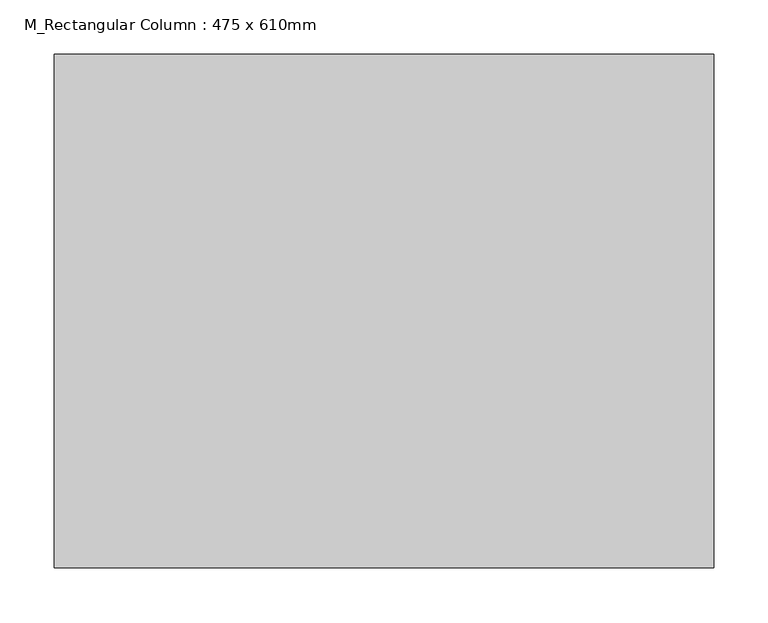
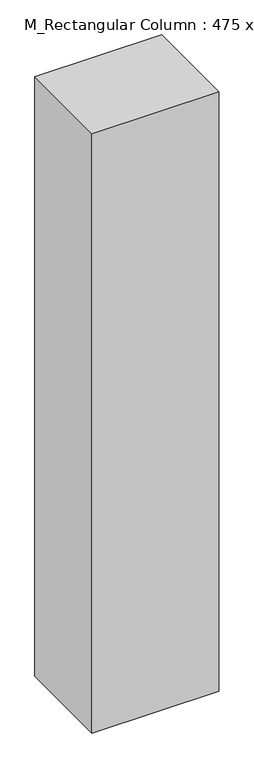
"""IFC4 building model written with IfcOpenShell, lengths in millimetres: column geometry, M_Rectangular Column : 475 x 610mm."""

from ifc_helpers import new_model, si_unit, origin, origin_with_axes, place, context, project, spatial, polyline, outline, extrude, source, transform, mapped, element, save


def m_rectangular_column_475_x_610mm_5ff218ee(model_context):
    return source(origin(), model_context, "Body", "SweptSolid", [
        extrude(outline(polyline([(305.0, 237.5), (305.0, -237.5), (-305.0, -237.5), (-305.0, 237.5), (305.0, 237.5)])), origin_with_axes(), (0.0, 0.0, 1.0), 3048.0),
    ])


if __name__ == "__main__":
    model = new_model("IFC4")
    model_context = context("Model", 3, world=origin())
    ifc_project = project(units=[si_unit("LENGTHUNIT", "METRE", prefix="MILLI")], contexts=[model_context])
    site = spatial("IfcSite", under=ifc_project)
    building = spatial("IfcBuilding", under=site)
    placement = place(None, origin())
    m_rectangular_column_475_x_610mm_shape = m_rectangular_column_475_x_610mm_5ff218ee(model_context)
    element("IfcColumn", 1, ObjectType="M_Rectangular Column : 475 x 610mm", at=placement, inside=building, context=model_context, shape_type="MappedRepresentation", body=[
        mapped(m_rectangular_column_475_x_610mm_shape, transform((0.0, 0.0, 0.0), x_axis=(1.0, 0.0, 0.0), y_axis=(0.0, 1.0, 0.0), z_axis=(0.0, 0.0, 1.0))),
    ])
    save(model, "model.ifc")

# Revit data of these elements
# Type "M_Rectangular Column : 475 x 610mm"
#   Depth = 1' - 6.70079"
#   Offset Base = 0' - 0"
#   Offset Top = 0' - 0"
#   Width = 2' - 0.01575"
#   Material = none
